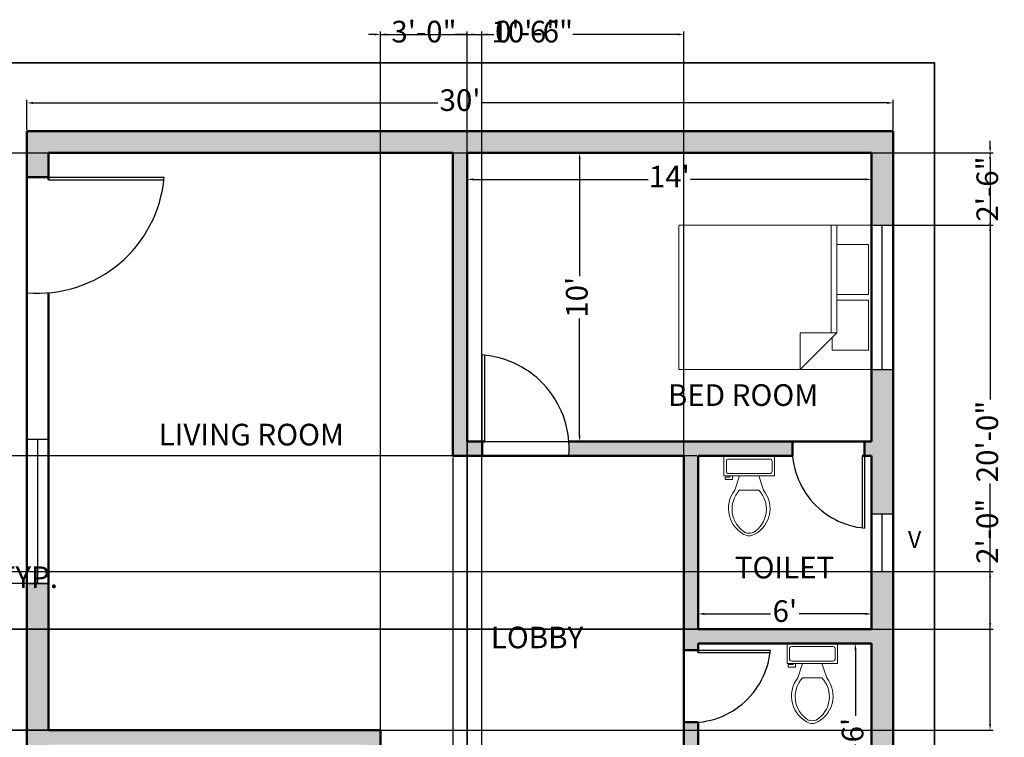
# Model space of a CAD drawing. Units: inches. Extents: x 2463 to 3327, y 6994 to 7582.
# Tile 5 of 5: x 2917 to 3327, y 7269 to 7567. Entities that reach past the tile are written whole.
import ezdxf

# ---------------------------------------------------------------- set-up
doc = ezdxf.new("R2010")
doc.units = ezdxf.units.IN
for name, color, linetype, lineweight in [('A-ANNO-DIMS', 2, 'Continuous', 18), ('A-ANNO-TEXT', 7, 'Continuous', 18), ('A-ANNO-TTLB', 7, 'Continuous', 35), ('A-AREA-IDEN', 3, 'Continuous', 25), ('A-DOOR', 4, 'Continuous', 25), ('A-FLOR-FIXT', 8, 'Continuous', 18), ('A-FURN', 8, 'Continuous', 18), ('A-GLAZ', 4, 'Continuous', 25), ('A-WALL', 7, 'Continuous', 50), ('A-WALL-PATT', 252, 'Continuous', 13)]:
    doc.layers.add(name, color=color, linetype=linetype, lineweight=lineweight)
doc.styles.get("Standard").update_dxf_attribs({"font": 'times.ttf'})
doc.dimstyles.new('ISO-25', dxfattribs={"dimtxt": 9, "dimasz": 2.5, "dimexe": 1.25, "dimexo": 0.625, "dimgap": 2, "dimtad": 0, "dimdec": 1, "dimlunit": 4, "dimtxsty": 'Standard', "dimcen": 2.5, "dimadec": 0, "dimazin": 0, "dimtfac": 1, "dimtdec": 1, "dimtmove": 0, "dimatfit": 3, "dimfxl": 1, "dimarcsym": 0})

# ---------------------------------------------------------------- blocks, each defined once
blk = doc.blocks.new('*D15')
at = {"layer": 'A-ANNO-DIMS', "color": 0, "lineweight": -2, "transparency": 16777216}
for p, q in [((3103.42, 7511.2), (3103.42, 7499.6)), ((3271.42, 7511.2), (3271.42, 7499.6)), ((3105.92, 7500.85), (3178.64, 7500.85)), ((3268.92, 7500.85), (3196.2, 7500.85))]:
    blk.add_line(p, q, dxfattribs=at)
at = {"layer": 'A-ANNO-DIMS', "color": 0, "transparency": 16777216}
for points in [[(3105.92, 7501.27), (3105.92, 7500.43), (3103.42, 7500.85)], [(3268.92, 7501.27), (3268.92, 7500.43), (3271.42, 7500.85)]]:
    blk.add_solid(points, dxfattribs=at)
at = {"layer": 'Defpoints', "color": 0, "transparency": 16777216}
for p in [(3103.42, 7511.83), (3271.42, 7511.83), (3271.42, 7500.85)]:
    blk.add_point(p, dxfattribs=at)
at = {"layer": 'A-ANNO-DIMS', "color": 0, "transparency": 16777216, "insert": (3187.42, 7500.85), "char_height": 9, "attachment_point": 5}
blk.add_mtext("14'", dxfattribs=at)
blk = doc.blocks.new('*D16')
at = {"layer": 'A-ANNO-DIMS', "color": 0, "lineweight": -2, "transparency": 16777216}
for p, q in [((3104.05, 7511.83), (3151.36, 7511.83)), ((3150.11, 7509.33), (3150.11, 7460.61)), ((3150.11, 7394.33), (3150.11, 7443.04)), ((3104.05, 7391.83), (3151.36, 7391.83))]:
    blk.add_line(p, q, dxfattribs=at)
at = {"layer": 'A-ANNO-DIMS', "color": 0, "transparency": 16777216}
for points in [[(3149.69, 7509.33), (3150.53, 7509.33), (3150.11, 7511.83)], [(3149.69, 7394.33), (3150.53, 7394.33), (3150.11, 7391.83)]]:
    blk.add_solid(points, dxfattribs=at)
at = {"layer": 'Defpoints', "color": 0, "transparency": 16777216}
for p in [(3103.42, 7511.83), (3103.42, 7391.83), (3150.11, 7391.83)]:
    blk.add_point(p, dxfattribs=at)
at = {"layer": 'A-ANNO-DIMS', "color": 0, "transparency": 16777216, "insert": (3150.11, 7451.83), "char_height": 9, "attachment_point": 5, "rotation": 90}
blk.add_mtext("10'", dxfattribs=at)
blk = doc.blocks.new('*D17')
at = {"layer": 'A-ANNO-DIMS', "color": 0, "lineweight": -2, "transparency": 16777216}
for p, q in [((3270.8, 7307.83), (3263.49, 7307.83)), ((3264.74, 7305.33), (3264.74, 7277.78)), ((3264.74, 7238.33), (3264.74, 7265.87)), ((3270.8, 7235.83), (3263.49, 7235.83))]:
    blk.add_line(p, q, dxfattribs=at)
at = {"layer": 'A-ANNO-DIMS', "color": 0, "transparency": 16777216}
for points in [[(3264.33, 7305.33), (3265.16, 7305.33), (3264.74, 7307.83)], [(3264.33, 7238.33), (3265.16, 7238.33), (3264.74, 7235.83)]]:
    blk.add_solid(points, dxfattribs=at)
at = {"layer": 'Defpoints', "color": 0, "transparency": 16777216}
for p in [(3264.74, 7307.83), (3271.42, 7307.83), (3271.42, 7235.83)]:
    blk.add_point(p, dxfattribs=at)
at = {"layer": 'A-ANNO-DIMS', "color": 0, "transparency": 16777216, "insert": (3264.74, 7271.83), "char_height": 9, "attachment_point": 5, "rotation": 90}
blk.add_mtext("6'", dxfattribs=at)
blk = doc.blocks.new('Bed - Queen')
for p, q in [((0, -80.00003), (0, 0)), ((0, 0), (59.99999, 0)), ((59.99999, 0), (59.99999, -80.00003)), ((7.99999, -1.2), (28.79998, -1.2)), ((7.99999, -14.4), (7.99999, -1.2)), ((28.79998, -1.2), (28.79998, -14.4)), ((31.19999, -1.2), (51.99999, -1.2)), ((31.19999, -14.4), (31.19999, -1.2)), ((51.99999, -1.2), (51.99999, -16.4)), ((0, -14.4), (44.8, -14.4)), ((59.99999, -29.6), (44.8, -14.4)), ((44.8, -14.4), (44.8, -29.6)), ((44.8, -16.8), (0, -16.8)), ((51.99999, -16.4), (46.79936, -16.4)), ((44.8, -29.6), (59.99999, -29.6)), ((59.99999, -80.00003), (0, -80.00003))]:
    blk.add_line(p, q)
blk = doc.blocks.new('*D18')
at = {"layer": 'A-ANNO-DIMS', "color": 0, "lineweight": -2, "transparency": 16777216}
for p, q in [((3199.42, 7314.45), (3199.42, 7321.4)), ((3271.42, 7314.45), (3271.42, 7321.4)), ((3201.92, 7320.15), (3229.47, 7320.15)), ((3268.92, 7320.15), (3241.37, 7320.15))]:
    blk.add_line(p, q, dxfattribs=at)
at = {"layer": 'A-ANNO-DIMS', "color": 0, "transparency": 16777216}
for points in [[(3201.92, 7320.57), (3201.92, 7319.73), (3199.42, 7320.15)], [(3268.92, 7320.57), (3268.92, 7319.73), (3271.42, 7320.15)]]:
    blk.add_solid(points, dxfattribs=at)
at = {"layer": 'Defpoints', "color": 0, "transparency": 16777216}
for p in [(3271.42, 7320.15), (3199.42, 7313.83), (3271.42, 7313.83)]:
    blk.add_point(p, dxfattribs=at)
at = {"layer": 'A-ANNO-DIMS', "color": 0, "transparency": 16777216, "insert": (3235.42, 7320.15), "char_height": 9, "attachment_point": 5}
blk.add_mtext("6'", dxfattribs=at)
blk = doc.blocks.new('*U11')
for p, q in [((9.5, -6), (9.5, -2)), ((-8, -8.5), (-8, -8)), ((-7, -8), (-7, -9.5)), ((-4, -8), (-6, -14)), ((4, -8), (6, -14)), ((-10, -8.5), (-8, -8.5)), ((-10, -9.5), (-10, -8.5)), ((-7, -9.5), (-10, -9.5)), ((4, -14), (-4, -14))]:
    blk.add_line(p, q)
blk.add_lwpolyline([(10.5, -8), (10.5, 0), (-10.5, 0), (-10.5, -8)], close=True)
for points in [[(-9.5, -2), (-9.5, -6)], [(8.5, -1), (-8.5, -1)], [(-8.5, -7), (8.5, -7)]]:
    blk.add_lwpolyline(points)
for centre, radius, start, end in [((-8.62, -1.88), 0.884, 81.8699, 188.1301), ((8.62, -1.88), 0.884, 351.8699, 98.1301), ((-8.62, -6.12), 0.884, 171.8699, 278.1301), ((8.62, -6.12), 0.884, 261.8699, 8.1301), ((3.52, -21.58), 12.17, 141.4691, 247.9714), ((4.2, -21.82), 11.33, 136.3677, 238.9468), ((-3.52, -21.58), 12.17, 292.0284, 38.5307), ((-4.2, -21.82), 11.33, 301.053, 43.6321), ((0, -27.88), 4, 245.7318, 294.2682), ((0, -29), 4, 254.8605, 285.1395)]:
    blk.add_arc(centre, radius, start, end)
blk = doc.blocks.new('*D25')
at = {"layer": 'A-ANNO-DIMS', "color": 0, "lineweight": -2, "transparency": 16777216}
for p, q in [((2920.42, 7521.45), (2920.42, 7533.89)), ((2922.92, 7532.64), (3091.13, 7532.64)), ((3277.92, 7532.64), (3109.71, 7532.64)), ((3280.42, 7521.45), (3280.42, 7533.89))]:
    blk.add_line(p, q, dxfattribs=at)
at = {"layer": 'A-ANNO-DIMS', "color": 0, "transparency": 16777216}
for points in [[(2922.92, 7533.06), (2922.92, 7532.22), (2920.42, 7532.64)], [(3277.92, 7533.06), (3277.92, 7532.22), (3280.42, 7532.64)]]:
    blk.add_solid(points, dxfattribs=at)
at = {"layer": 'Defpoints', "color": 0, "transparency": 16777216}
for p in [(3280.42, 7532.64), (2920.42, 7520.83), (3280.42, 7520.83)]:
    blk.add_point(p, dxfattribs=at)
at = {"layer": 'A-ANNO-DIMS', "color": 0, "transparency": 16777216, "insert": (3100.42, 7532.64), "char_height": 9, "attachment_point": 5}
blk.add_mtext("30'", dxfattribs=at)
blk = doc.blocks.new('DOOR-36')
for p, q in [((0, 6), (0, 42)), ((1, 6), (1, 41.91))]:
    blk.add_line(p, q)
blk.add_arc((-3, 3), 39.12, 355.6013, 85.6013)
blk = doc.blocks.new('DOOR-30')
for p, q in [((29.14, 30), (29.14, 0)), ((30.14, 30), (30.14, 0))]:
    blk.add_line(p, q)
blk.add_arc((33.14, 33), 33.14, 174.8056, 264.8056)
blk = doc.blocks.new('DOOR-48')
for p, q in [((9, 48.19), (57, 48.19)), ((9, 47.19), (56.91, 47.19))]:
    blk.add_line(p, q)
blk.add_arc((4.5, 52.69), 52.69, 265.1009, 355.1009)
blk = doc.blocks.new('WIN-60')
for p, q in [((9, 60), (0, 60)), ((4.5, 60), (4.5, 0)), ((9, 0), (0, 0))]:
    blk.add_line(p, q)
blk = doc.blocks.new('WIN-24')
for p, q in [((9, 24), (0, 24)), ((4.5, 24), (4.5, 0)), ((9, 0), (0, 0))]:
    blk.add_line(p, q)
blk = doc.blocks.new('*D40')
at = {"layer": 'A-ANNO-DIMS', "color": 0, "lineweight": -2, "transparency": 16777216}
for p, q in [((2864.43, 7337.2), (2864.43, 7332.98)), ((2866.93, 7334.23), (2870.93, 7334.23)), ((2873.43, 7337.2), (2873.43, 7332.98)), ((2873.43, 7334.23), (2875.93, 7334.23))]:
    blk.add_line(p, q, dxfattribs=at)
at = {"layer": 'A-ANNO-DIMS', "color": 0, "transparency": 16777216}
for points in [[(2866.93, 7334.64), (2866.93, 7333.81), (2864.43, 7334.23)], [(2870.93, 7334.64), (2870.93, 7333.81), (2873.43, 7334.23)]]:
    blk.add_solid(points, dxfattribs=at)
at = {"layer": 'Defpoints', "color": 0, "transparency": 16777216}
for p in [(2864.43, 7337.83), (2873.43, 7337.83), (2873.43, 7334.23)]:
    blk.add_point(p, dxfattribs=at)
at = {"layer": 'A-ANNO-DIMS', "color": 0, "transparency": 16777216, "insert": (2905.86, 7334.23), "char_height": 9, "attachment_point": 5}
blk.add_mtext('0\'-9" TYP.', dxfattribs=at)
blk = doc.blocks.new('*D51')
at = {"layer": 'A-ANNO-DIMS', "color": 0, "lineweight": -2, "transparency": 16777216}
for p, q in [((2523.06, 7511.83), (3321.97, 7511.83)), ((3320.72, 7509.33), (3320.72, 7409.33)), ((3320.72, 7274.33), (3320.72, 7374.32)), ((2523.06, 7271.83), (3321.97, 7271.83))]:
    blk.add_line(p, q, dxfattribs=at)
at = {"layer": 'A-ANNO-DIMS', "color": 0, "transparency": 16777216}
for points in [[(3320.31, 7509.33), (3321.14, 7509.33), (3320.72, 7511.83)], [(3320.31, 7274.33), (3321.14, 7274.33), (3320.72, 7271.83)]]:
    blk.add_solid(points, dxfattribs=at)
at = {"layer": 'Defpoints', "color": 0, "transparency": 16777216}
for p in [(2522.43, 7511.83), (2522.43, 7271.83), (3320.72, 7271.83)]:
    blk.add_point(p, dxfattribs=at)
at = {"layer": 'A-ANNO-DIMS', "color": 0, "transparency": 16777216, "insert": (3320.72, 7391.83), "char_height": 9, "attachment_point": 5, "rotation": 90}
blk.add_mtext('20\'-0"', dxfattribs=at)
blk = doc.blocks.new('*D65')
at = {"layer": 'A-ANNO-DIMS', "color": 0, "lineweight": -2, "transparency": 16777216}
for p, q in [((2865.06, 7337.83), (3321.97, 7337.83)), ((3320.72, 7337.83), (3320.72, 7340.33)), ((3320.72, 7316.33), (3320.72, 7335.33)), ((2865.06, 7313.83), (3321.97, 7313.83))]:
    blk.add_line(p, q, dxfattribs=at)
at = {"layer": 'A-ANNO-DIMS', "color": 0, "transparency": 16777216}
for points in [[(3320.31, 7335.33), (3321.14, 7335.33), (3320.72, 7337.83)], [(3320.31, 7316.33), (3321.14, 7316.33), (3320.72, 7313.83)]]:
    blk.add_solid(points, dxfattribs=at)
at = {"layer": 'Defpoints', "color": 0, "transparency": 16777216}
for p in [(2864.43, 7337.83), (3320.72, 7337.83), (2864.43, 7313.83)]:
    blk.add_point(p, dxfattribs=at)
at = {"layer": 'A-ANNO-DIMS', "color": 0, "transparency": 16777216, "insert": (3320.72, 7354.51), "char_height": 9, "attachment_point": 5, "rotation": 90}
blk.add_mtext('2\'-0"', dxfattribs=at)
blk = doc.blocks.new('*D68')
at = {"layer": 'A-ANNO-DIMS', "color": 0, "lineweight": -2, "transparency": 16777216}
for p, q in [((3103.42, 7391.2), (3103.42, 6999.28)), ((3097.42, 7385.2), (3097.42, 6999.28)), ((3094.92, 7000.53), (3092.42, 7000.53)), ((3097.42, 7000.53), (3103.42, 7000.53)), ((3105.92, 7000.53), (3108.42, 7000.53))]:
    blk.add_line(p, q, dxfattribs=at)
at = {"layer": 'A-ANNO-DIMS', "color": 0, "transparency": 16777216}
for points in [[(3094.92, 7000.94), (3094.92, 7000.11), (3097.42, 7000.53)], [(3105.92, 7000.94), (3105.92, 7000.11), (3103.42, 7000.53)]]:
    blk.add_solid(points, dxfattribs=at)
at = {"layer": 'Defpoints', "color": 0, "transparency": 16777216}
for p in [(3103.42, 7391.83), (3097.42, 7385.83), (3103.42, 7000.53)]:
    blk.add_point(p, dxfattribs=at)
at = {"layer": 'A-ANNO-DIMS', "color": 0, "transparency": 16777216, "insert": (3122.51, 7000.53), "char_height": 9, "attachment_point": 5}
blk.add_mtext('0\'-6"', dxfattribs=at)
blk = doc.blocks.new('*D69')
at = {"layer": 'A-ANNO-DIMS', "color": 0, "lineweight": -2, "transparency": 16777216}
for p, q in [((3198.8, 7385.83), (2471.88, 7385.83)), ((2473.13, 7383.33), (2473.13, 7363.87)), ((2473.13, 7316.33), (2473.13, 7335.79)), ((3198.8, 7313.83), (2471.88, 7313.83))]:
    blk.add_line(p, q, dxfattribs=at)
at = {"layer": 'A-ANNO-DIMS', "color": 0, "transparency": 16777216}
for points in [[(2472.71, 7383.33), (2473.55, 7383.33), (2473.13, 7385.83)], [(2472.71, 7316.33), (2473.55, 7316.33), (2473.13, 7313.83)]]:
    blk.add_solid(points, dxfattribs=at)
at = {"layer": 'Defpoints', "color": 0, "transparency": 16777216}
for p in [(3199.42, 7385.83), (2473.13, 7313.83), (3199.42, 7313.83)]:
    blk.add_point(p, dxfattribs=at)
at = {"layer": 'A-ANNO-DIMS', "color": 0, "transparency": 16777216, "insert": (2473.13, 7349.83), "char_height": 9, "attachment_point": 5, "rotation": 90}
blk.add_mtext('6\'-0"', dxfattribs=at)
blk = doc.blocks.new('*D70')
at = {"layer": 'A-ANNO-DIMS', "color": 0, "lineweight": -2, "transparency": 16777216}
for p, q in [((2930.05, 7511.83), (3321.97, 7511.83)), ((3320.72, 7509.33), (3320.72, 7409.33)), ((3320.72, 7274.33), (3320.72, 7374.32)), ((2930.05, 7271.83), (3321.97, 7271.83))]:
    blk.add_line(p, q, dxfattribs=at)
at = {"layer": 'A-ANNO-DIMS', "color": 0, "transparency": 16777216}
for points in [[(3320.31, 7509.33), (3321.14, 7509.33), (3320.72, 7511.83)], [(3320.31, 7274.33), (3321.14, 7274.33), (3320.72, 7271.83)]]:
    blk.add_solid(points, dxfattribs=at)
at = {"layer": 'Defpoints', "color": 0, "transparency": 16777216}
for p in [(2929.42, 7511.83), (2929.42, 7271.83), (3320.72, 7271.83)]:
    blk.add_point(p, dxfattribs=at)
at = {"layer": 'A-ANNO-DIMS', "color": 0, "transparency": 16777216, "insert": (3320.72, 7391.83), "char_height": 9, "attachment_point": 5, "rotation": 90}
blk.add_mtext('20\'-0"', dxfattribs=at)
blk = doc.blocks.new('*D71')
at = {"layer": 'A-ANNO-DIMS', "color": 0, "lineweight": -2, "transparency": 16777216}
for p, q in [((3067.42, 7272.45), (3067.42, 7562.38)), ((3069.92, 7561.13), (3113.55, 7561.13)), ((3190.92, 7561.13), (3147.29, 7561.13)), ((3193.42, 7230.45), (3193.42, 7562.38))]:
    blk.add_line(p, q, dxfattribs=at)
at = {"layer": 'A-ANNO-DIMS', "color": 0, "transparency": 16777216}
for points in [[(3069.92, 7561.54), (3069.92, 7560.71), (3067.42, 7561.13)], [(3190.92, 7561.54), (3190.92, 7560.71), (3193.42, 7561.13)]]:
    blk.add_solid(points, dxfattribs=at)
at = {"layer": 'Defpoints', "color": 0, "transparency": 16777216}
for p in [(3193.42, 7561.13), (3067.42, 7271.83), (3193.42, 7229.83)]:
    blk.add_point(p, dxfattribs=at)
at = {"layer": 'A-ANNO-DIMS', "color": 0, "transparency": 16777216, "insert": (3130.42, 7561.13), "char_height": 9, "attachment_point": 5}
blk.add_mtext('10\'-6"', dxfattribs=at)
blk = doc.blocks.new('*D73')
at = {"layer": 'A-ANNO-DIMS', "color": 0, "lineweight": -2, "transparency": 16777216}
for p, q in [((3064.92, 7561.13), (3062.42, 7561.13)), ((3067.42, 7180.45), (3067.42, 7562.38)), ((3067.42, 7561.13), (3071.37, 7561.13)), ((3103.42, 7561.13), (3099.48, 7561.13)), ((3103.42, 7190.45), (3103.42, 7562.38)), ((3105.92, 7561.13), (3108.42, 7561.13))]:
    blk.add_line(p, q, dxfattribs=at)
at = {"layer": 'A-ANNO-DIMS', "color": 0, "transparency": 16777216}
for points in [[(3064.92, 7561.54), (3064.92, 7560.71), (3067.42, 7561.13)], [(3105.92, 7561.54), (3105.92, 7560.71), (3103.42, 7561.13)]]:
    blk.add_solid(points, dxfattribs=at)
at = {"layer": 'Defpoints', "color": 0, "transparency": 16777216}
for p in [(3103.42, 7561.13), (3103.42, 7189.83), (3067.42, 7179.83)]:
    blk.add_point(p, dxfattribs=at)
at = {"layer": 'A-ANNO-DIMS', "color": 0, "transparency": 16777216, "insert": (3085.42, 7561.13), "char_height": 9, "attachment_point": 5}
blk.add_mtext('3\'-0"', dxfattribs=at)
blk = doc.blocks.new('*D74')
at = {"layer": 'A-ANNO-DIMS', "color": 0, "lineweight": -2, "transparency": 16777216}
for p, q in [((3100.92, 7561.13), (3098.42, 7561.13)), ((3103.42, 7190.45), (3103.42, 7562.38)), ((3103.42, 7561.13), (3109.42, 7561.13)), ((3109.42, 7190.45), (3109.42, 7562.38)), ((3111.92, 7561.13), (3114.42, 7561.13))]:
    blk.add_line(p, q, dxfattribs=at)
at = {"layer": 'A-ANNO-DIMS', "color": 0, "transparency": 16777216}
for points in [[(3100.92, 7561.54), (3100.92, 7560.71), (3103.42, 7561.13)], [(3111.92, 7561.54), (3111.92, 7560.71), (3109.42, 7561.13)]]:
    blk.add_solid(points, dxfattribs=at)
at = {"layer": 'Defpoints', "color": 0, "transparency": 16777216}
for p in [(3109.42, 7561.13), (3103.42, 7189.83), (3109.42, 7189.83)]:
    blk.add_point(p, dxfattribs=at)
at = {"layer": 'A-ANNO-DIMS', "color": 0, "transparency": 16777216, "insert": (3128.51, 7561.13), "char_height": 9, "attachment_point": 5}
blk.add_mtext('0\'-6"', dxfattribs=at)
blk = doc.blocks.new('*D78')
at = {"layer": 'A-ANNO-DIMS', "color": 0, "lineweight": -2, "transparency": 16777216}
for p, q in [((2928.8, 7332.77), (2471.88, 7332.77)), ((2473.13, 7330.27), (2473.13, 7316.3)), ((2473.13, 7274.33), (2473.13, 7288.29)), ((2928.8, 7271.83), (2471.88, 7271.83))]:
    blk.add_line(p, q, dxfattribs=at)
at = {"layer": 'A-ANNO-DIMS', "color": 0, "transparency": 16777216}
for points in [[(2472.71, 7330.27), (2473.55, 7330.27), (2473.13, 7332.77)], [(2472.71, 7274.33), (2473.55, 7274.33), (2473.13, 7271.83)]]:
    blk.add_solid(points, dxfattribs=at)
at = {"layer": 'Defpoints', "color": 0, "transparency": 16777216}
for p in [(2473.13, 7332.77), (2929.42, 7332.77), (2929.42, 7271.83)]:
    blk.add_point(p, dxfattribs=at)
at = {"layer": 'A-ANNO-DIMS', "color": 0, "transparency": 16777216, "insert": (2473.13, 7302.3), "char_height": 9, "attachment_point": 5, "rotation": 90}
blk.add_mtext('5\'-1"', dxfattribs=at)
blk = doc.blocks.new('*D79')
at = {"layer": 'A-ANNO-DIMS', "color": 0, "lineweight": -2, "transparency": 16777216}
for p, q in [((3320.72, 7514.33), (3320.72, 7516.83)), ((3272.05, 7511.83), (3321.97, 7511.83)), ((3320.72, 7511.83), (3320.72, 7511.01)), ((3272.05, 7481.83), (3321.97, 7481.83)), ((3320.72, 7481.83), (3320.72, 7482.64)), ((3320.72, 7479.33), (3320.72, 7476.83))]:
    blk.add_line(p, q, dxfattribs=at)
at = {"layer": 'A-ANNO-DIMS', "color": 0, "transparency": 16777216}
for points in [[(3320.31, 7514.33), (3321.14, 7514.33), (3320.72, 7511.83)], [(3320.31, 7479.33), (3321.14, 7479.33), (3320.72, 7481.83)]]:
    blk.add_solid(points, dxfattribs=at)
at = {"layer": 'Defpoints', "color": 0, "transparency": 16777216}
for p in [(3271.42, 7511.83), (3271.42, 7481.83), (3320.72, 7481.83)]:
    blk.add_point(p, dxfattribs=at)
at = {"layer": 'A-ANNO-DIMS', "color": 0, "transparency": 16777216, "insert": (3320.72, 7496.83), "char_height": 9, "attachment_point": 5, "rotation": 90}
blk.add_mtext('2\'-6"', dxfattribs=at)
blk = doc.blocks.new('*D80')
at = {"layer": 'A-ANNO-DIMS', "color": 0, "lineweight": -2, "transparency": 16777216}
for p, q in [((3272.05, 7337.83), (3321.97, 7337.83)), ((3320.72, 7337.83), (3320.72, 7340.33)), ((3320.72, 7316.33), (3320.72, 7335.33)), ((3272.05, 7313.83), (3321.97, 7313.83))]:
    blk.add_line(p, q, dxfattribs=at)
at = {"layer": 'A-ANNO-DIMS', "color": 0, "transparency": 16777216}
for points in [[(3320.31, 7335.33), (3321.14, 7335.33), (3320.72, 7337.83)], [(3320.31, 7316.33), (3321.14, 7316.33), (3320.72, 7313.83)]]:
    blk.add_solid(points, dxfattribs=at)
at = {"layer": 'Defpoints', "color": 0, "transparency": 16777216}
for p in [(3271.42, 7337.83), (3320.72, 7337.83), (3271.42, 7313.83)]:
    blk.add_point(p, dxfattribs=at)
at = {"layer": 'A-ANNO-DIMS', "color": 0, "transparency": 16777216, "insert": (3320.72, 7354.51), "char_height": 9, "attachment_point": 5, "rotation": 90}
blk.add_mtext('2\'-0"', dxfattribs=at)

msp = doc.modelspace()

# ---------------------------------------------------------------- hatches: boundary and pattern name
at = {"layer": 'A-WALL-PATT'}
h = msp.add_hatch(color=256, dxfattribs=at)
h.dxf.hatch_style = 1
h.paths.add_polyline_path([(2522.43, 7511.83), (2690.43, 7511.83), (2690.43, 7385.83), (2696.43, 7385.83), (2702.68, 7385.83), (2702.68, 7391.83), (2696.43, 7391.83), (2696.43, 7511.83), (2864.43, 7511.83), (2864.43, 7481.83), (2873.43, 7481.83), (2873.43, 7520.83), (2513.43, 7520.83), (2513.43, 7501.71), (2522.43, 7501.71)])
h.paths.add_polyline_path([(2522.43, 7453.71, -0.042779), (2513.43, 7453.71), (2513.43, 7392.77), (2522.43, 7392.77)], flags=0)
h.paths.add_polyline_path([(2522.43, 7332.77), (2513.43, 7332.77), (2513.43, 7226.83), (2522.43, 7226.83), (2522.43, 7265.83), (2654.43, 7265.83), (2654.43, 7263.42), (2660.43, 7263.42), (2660.43, 7271.83), (2522.43, 7271.83)])
h.paths.add_polyline_path([(2873.43, 7421.83), (2864.43, 7421.83), (2864.43, 7391.83), (2861.59, 7391.83), (2861.59, 7385.83), (2864.43, 7385.83), (2864.43, 7361.83), (2873.43, 7361.83)])
h.paths.add_polyline_path([(2792.43, 7385.83), (2831.59, 7385.83, -0.045361), (2831.59, 7391.83), (2738.68, 7391.83, -0.038405), (2738.68, 7385.83), (2786.43, 7385.83), (2786.43, 7313.83), (2786.43, 7307.83), (2786.43, 7305.07), (2792.43, 7305.07), (2792.43, 7307.83), (2864.43, 7307.83), (2864.43, 7235.83), (2792.43, 7235.83), (2792.43, 7275.07, -0.045361), (2786.43, 7275.07), (2786.43, 7235.83), (2786.43, 7229.83), (2864.43, 7229.83), (2864.43, 7169.83), (2873.43, 7169.83), (2873.43, 7337.83), (2864.43, 7337.83), (2864.43, 7313.83), (2792.43, 7313.83)])
h.paths.add_polyline_path([(2873.43, 7109.83), (2864.43, 7109.83), (2864.43, 7049.83), (2834.43, 7049.83), (2834.43, 7040.83), (2873.43, 7040.83)])
h.paths.add_polyline_path([(2774.43, 7049.83), (2744.43, 7049.83), (2744.43, 7199.83), (2738.43, 7199.83), (2738.43, 7049.83), (2723.43, 7049.83), (2723.43, 7040.83), (2774.43, 7040.83)])
h.paths.add_polyline_path([(2675.43, 7049.83), (2660.43, 7049.83), (2660.43, 7121.83), (2660.43, 7127.83), (2660.43, 7227.42, -0.038405), (2654.43, 7227.42), (2654.43, 7127.83), (2651.08, 7127.83), (2651.08, 7121.83), (2654.43, 7121.83), (2654.43, 7049.83), (2522.43, 7049.83), (2522.43, 7073.83), (2513.43, 7073.83), (2513.43, 7040.83), (2675.43, 7040.83)])
h.paths.add_polyline_path([(2621.08, 7127.83), (2522.43, 7127.83), (2522.43, 7166.83), (2513.43, 7166.83), (2513.43, 7097.83), (2522.43, 7097.83), (2522.43, 7121.83), (2621.08, 7121.83, -0.045361)], flags=17)
h.paths.add_polyline_path([(3280.42, 7520.83), (2920.42, 7520.83), (2920.42, 7501.71), (2929.42, 7501.71), (2929.42, 7511.83), (3097.42, 7511.83), (3097.42, 7385.83), (3103.42, 7385.83), (3109.67, 7385.83), (3109.67, 7391.83), (3103.42, 7391.83), (3103.42, 7511.83), (3271.42, 7511.83), (3271.42, 7481.83), (3280.42, 7481.83)])
h.paths.add_polyline_path([(3280.42, 7421.83), (3271.42, 7421.83), (3271.42, 7391.83), (3268.58, 7391.83), (3268.58, 7385.83), (3271.42, 7385.83), (3271.42, 7361.83), (3280.42, 7361.83)])
h.paths.add_polyline_path([(3238.58, 7391.83), (3145.67, 7391.83, -0.038405), (3145.67, 7385.83), (3193.42, 7385.83), (3193.42, 7313.83), (3193.42, 7307.83), (3193.42, 7305.07), (3199.42, 7305.07), (3199.42, 7307.83), (3271.42, 7307.83), (3271.42, 7235.83), (3199.42, 7235.83), (3193.42, 7235.83), (3193.42, 7229.83), (3271.42, 7229.83), (3280.42, 7229.83), (3280.42, 7337.83), (3271.42, 7337.83), (3271.42, 7313.83), (3199.42, 7313.83), (3199.42, 7385.83), (3238.58, 7385.83, -0.045361)])
h.paths.add_polyline_path([(3199.42, 7275.07, -0.045361), (3193.42, 7275.07), (3193.42, 7235.83), (3199.42, 7235.83)], flags=17)
h.paths.add_polyline_path([(3193.42, 7235.83), (3145.42, 7235.83), (3145.42, 7227.44), (3151.42, 7227.44), (3151.42, 7229.83), (3193.42, 7229.83)])
h.paths.add_polyline_path([(3151.42, 7199.83, -0.044871), (3145.42, 7199.83), (3145.42, 7049.83), (3130.42, 7049.83), (3130.42, 7040.83), (3151.42, 7040.83), (3151.42, 7049.83)])
h.paths.add_polyline_path([(3082.42, 7049.83), (3067.42, 7049.83), (3067.42, 7121.83), (3067.42, 7127.83), (3067.42, 7227.42, -0.038405), (3061.42, 7227.42), (3061.42, 7127.83), (3058.07, 7127.83), (3058.07, 7121.83), (3061.42, 7121.83), (3061.42, 7049.83), (2929.42, 7049.83), (2929.42, 7073.83), (2920.42, 7073.83), (2920.42, 7040.83), (3082.42, 7040.83)])
h.paths.add_polyline_path([(3028.07, 7121.83), (2997.56, 7121.83), (2997.56, 7113.83), (2991.06, 7113.83), (2993.06, 7107.83, -0.501323), (2988.1, 7088.96, -0.132891), (2986.01, 7088.96, -0.501317), (2981.06, 7107.83), (2983.06, 7113.83), (2980.06, 7113.83), (2980.06, 7112.33), (2977.06, 7112.33), (2977.06, 7113.83), (2976.56, 7113.83), (2976.56, 7121.83), (2929.42, 7121.83), (2929.42, 7097.83), (2920.42, 7097.83), (2920.42, 7166.83), (2929.42, 7166.83), (2929.42, 7127.83), (3028.07, 7127.83, 0.045361)], flags=17)
h.paths.add_polyline_path([(2995.56, 7120.83, -0.414214), (2996.56, 7120.08), (2996.56, 7115.83, -0.414214), (2995.81, 7114.83), (2978.56, 7114.83, -0.414214), (2977.56, 7115.58), (2977.56, 7119.83, -0.414214), (2978.31, 7120.83)], flags=16)
h.paths.add_polyline_path([(2988.7, 7090.3, -0.215004), (2985.41, 7090.3, -0.48008), (2983.06, 7107.83), (2991.06, 7107.83, -0.48008)], flags=16)
h.paths.add_polyline_path([(2929.42, 7265.83), (3061.42, 7265.83), (3061.42, 7263.42), (3067.42, 7263.42), (3067.42, 7271.83), (2929.42, 7271.83), (2929.42, 7332.77), (2920.42, 7332.77), (2920.42, 7226.83), (2929.42, 7226.83)])
h.paths.add_polyline_path([(2929.42, 7453.71, -0.042779), (2920.42, 7453.71), (2920.42, 7392.77), (2929.42, 7392.77)], flags=0)

# ---------------------------------------------------------------- linework, layer by layer
at = {"layer": 'A-ANNO-TTLB'}
msp.add_lwpolyline([(2463.47, 7549.29), (3297.67, 7549.29), (3297.67, 7021.48), (2463.47, 7021.48)], close=True, dxfattribs=at)
at = {"layer": 'A-WALL'}
for p, q in [((2920.42, 7520.83), (3280.42, 7520.83)), ((2920.42, 7040.83), (2920.42, 7520.83)), ((3280.42, 7520.83), (3280.42, 7040.83)), ((2929.42, 7511.83), (3097.42, 7511.83)), ((2929.42, 7501.71), (2929.42, 7511.83)), ((3097.42, 7511.83), (3097.42, 7385.83)), ((3103.42, 7511.83), (3271.42, 7511.83)), ((3103.42, 7511.83), (3103.42, 7391.83)), ((3271.42, 7511.83), (3271.42, 7391.83)), ((2929.42, 7501.71), (2920.42, 7501.71)), ((2929.42, 7500.71), (2929.42, 7501.71)), ((2929.42, 7271.83), (2929.42, 7453.71)), ((3103.42, 7391.83), (3110.67, 7391.83)), ((3109.67, 7391.83), (3109.67, 7385.83)), ((3145.67, 7391.83), (3271.42, 7391.83)), ((3238.58, 7385.83), (3238.58, 7391.83)), ((3268.58, 7385.83), (3268.58, 7391.83)), ((3103.42, 7385.83), (3097.42, 7385.83)), ((3103.42, 7385.83), (3193.42, 7385.83)), ((3193.42, 7385.83), (3193.42, 7313.83)), ((3199.42, 7385.83), (3238.58, 7385.83)), ((3199.42, 7385.83), (3199.42, 7313.83)), ((3267.58, 7385.83), (3271.42, 7385.83)), ((3271.42, 7385.83), (3271.42, 7313.83)), ((3193.42, 7313.83), (3193.42, 7307.83)), ((3199.42, 7313.83), (3271.42, 7313.83)), ((3193.42, 7307.83), (3193.42, 7235.83)), ((3199.42, 7305.07), (3193.42, 7305.07)), ((3199.42, 7307.83), (3271.42, 7307.83)), ((3199.42, 7307.83), (3199.42, 7304.07)), ((3271.42, 7307.83), (3271.42, 7235.83)), ((3199.42, 7275.07), (3193.42, 7275.07)), ((3199.42, 7275.07), (3199.42, 7235.83)), ((3067.42, 7271.83), (2929.42, 7271.83)), ((3067.42, 7127.83), (3067.42, 7271.83))]:
    msp.add_line(p, q, dxfattribs=at)

# ---------------------------------------------------------------- block references
at = {"layer": 'A-DOOR'}
for name, p in [('DOOR-48', (2920.42, 7453.52)), ('DOOR-36', (3109.67, 7385.83)), ('DOOR-30', (3238.45, 7355.83))]:
    msp.add_blockref(name, p, dxfattribs=at)
at = {"layer": 'A-DOOR', "rotation": 90.02301063229471}
msp.add_blockref('DOOR-30', (3229.42, 7274.94), dxfattribs=at)
at = {"layer": 'A-FLOR-FIXT'}
for p in [(3220.61, 7385.55), (3246.82, 7307.55)]:
    msp.add_blockref('*U11', p, dxfattribs=at)
at = {"layer": 'A-FURN', "rotation": 270}
msp.add_blockref('Bed - Queen', (3271.42, 7481.83), dxfattribs=at)
at = {"layer": 'A-GLAZ', "rotation": 180}
for name, p in [('WIN-60', (3280.42, 7481.83)), ('WIN-60', (2929.42, 7392.77)), ('WIN-24', (3280.42, 7361.83))]:
    msp.add_blockref(name, p, dxfattribs=at)

# ---------------------------------------------------------------- texts
at = {"layer": 'A-ANNO-TEXT', "insert": (3275.15, 7354.57), "char_height": 7, "attachment_point": 1}
msp.add_mtext_dynamic_manual_height_columns('\\pxqc;{\\fTimes New Roman|b1|i0|c0|p18;V}', width=28.3852, gutter_width=12.5, heights=[0], dxfattribs=at)
at = {"layer": 'A-AREA-IDEN', "char_height": 9, "attachment_point": 1}
for s, width, insert in [('\\pxqc;{\\fTimes New Roman|b1|i0|c0|p18;BED ROOM}', 86.127, (3175, 7415.64)), ('\\pxqc;{\\fTimes New Roman|b1|i0|c0|p18;LIVING ROOM}', 122.533, (2952.42, 7399.21)), ('\\pxqc;{\\fTimes New Roman|b1|i0|c0|p18;TOILET}', 62.7452, (3203.92, 7343.91)), ('\\pxqc;{\\fTimes New Roman|b1|i0|c0|p18;LOBBY}', 90.7623, (3087.04, 7314.86))]:
    msp.add_mtext_dynamic_manual_height_columns(s, width=width, gutter_width=12.5, heights=[0], dxfattribs=dict(at, insert=insert))

# ---------------------------------------------------------------- dimensions: what is measured, and where the dimension line sits
at = {"layer": 'A-ANNO-DIMS'}
for base, p1, p2, override, picture, middle in [((3103.42, 7561.13), (3067.42, 7179.83), (3103.42, 7189.83), {"dimdec": 1, "dimlfac": 1, "dimrnd": 0, "dimzin": 1, "dimdsep": 46, "dimlunit": 4, "dimfrac": 2}, '*D73', (3085.42, 7561.13)), ((3193.42, 7561.13), (3067.42, 7271.83), (3193.42, 7229.83), {"dimdec": 1, "dimlfac": 1, "dimrnd": 0, "dimzin": 1, "dimdsep": 46, "dimlunit": 4, "dimfrac": 2}, '*D71', (3130.42, 7561.13)), ((3109.42, 7561.13), (3103.42, 7189.83), (3109.42, 7189.83), {"dimdec": 1, "dimlfac": 1, "dimrnd": 0, "dimzin": 1, "dimdsep": 46, "dimlunit": 4, "dimfrac": 2}, '*D74', (3128.51, 7561.13)), ((3280.42, 7532.64), (2920.42, 7520.83), (3280.42, 7520.83), {"dimclrd": 0, "dimclre": 0, "dimclrt": 0}, '*D25', (3100.42, 7532.64)), ((3271.42, 7500.85), (3103.42, 7511.83), (3271.42, 7511.83), {"dimclrd": 0, "dimclre": 0, "dimclrt": 0}, '*D15', (3187.42, 7500.85)), ((3103.42, 7000.53), (3097.42, 7385.83), (3103.42, 7391.83), {"dimdec": 1, "dimlfac": 1, "dimrnd": 0, "dimzin": 1, "dimdsep": 46, "dimlunit": 4, "dimfrac": 2}, '*D68', (3122.51, 7000.53)), ((3271.42, 7320.15), (3199.42, 7313.83), (3271.42, 7313.83), {"dimclrd": 0, "dimclre": 0, "dimclrt": 0}, '*D18', (3235.42, 7320.15))]:
    dim = msp.add_linear_dim(base=base, p1=p1, p2=p2, dimstyle='ISO-25', override=override, dxfattribs=at)
    dim.commit()
    dim.dimension.update_dxf_attribs({"geometry": picture, "text_midpoint": middle})
for base, p1, p2, override, picture, middle in [((3320.72, 7481.83), (3271.42, 7511.83), (3271.42, 7481.83), {"dimdec": 1, "dimlfac": 1, "dimrnd": 0, "dimzin": 1, "dimdsep": 46, "dimlunit": 4, "dimfrac": 2}, '*D79', (3320.72, 7496.83)), ((3320.72, 7271.83), (2522.43, 7511.83), (2522.43, 7271.83), {"dimdec": 1, "dimlfac": 1, "dimrnd": 0, "dimzin": 1, "dimdsep": 46, "dimlunit": 4, "dimfrac": 2}, '*D51', (3320.72, 7391.83)), ((3320.72, 7271.83), (2929.42, 7511.83), (2929.42, 7271.83), {"dimdec": 1, "dimlfac": 1, "dimrnd": 0, "dimzin": 1, "dimdsep": 46, "dimlunit": 4, "dimfrac": 2}, '*D70', (3320.72, 7391.83)), ((3150.11, 7391.83), (3103.42, 7511.83), (3103.42, 7391.83), {"dimclrd": 0, "dimclre": 0, "dimclrt": 0}, '*D16', (3150.11, 7451.83)), ((2473.13, 7313.83), (3199.42, 7385.83), (3199.42, 7313.83), {"dimdec": 1, "dimlfac": 1, "dimrnd": 0, "dimzin": 1, "dimdsep": 46, "dimlunit": 4, "dimfrac": 2}, '*D69', (2473.13, 7349.83)), ((3320.72, 7337.83), (2864.43, 7313.83), (2864.43, 7337.83), {"dimdec": 1, "dimlfac": 1, "dimrnd": 0, "dimzin": 1, "dimdsep": 46, "dimlunit": 4, "dimfrac": 2}, '*D65', (3320.72, 7354.51)), ((3320.72, 7337.83), (3271.42, 7313.83), (3271.42, 7337.83), {"dimdec": 1, "dimlfac": 1, "dimrnd": 0, "dimzin": 1, "dimdsep": 46, "dimlunit": 4, "dimfrac": 2}, '*D80', (3320.72, 7354.51)), ((2473.13, 7332.77), (2929.42, 7271.83), (2929.42, 7332.77), {"dimdec": 1, "dimlfac": 1, "dimrnd": 0, "dimzin": 1, "dimdsep": 46, "dimlunit": 4, "dimfrac": 2}, '*D78', (2473.13, 7302.3)), ((3264.74, 7307.83), (3271.42, 7235.83), (3271.42, 7307.83), {"dimclrd": 0, "dimclre": 0, "dimclrt": 0}, '*D17', (3264.74, 7271.83))]:
    dim = msp.add_linear_dim(base=base, p1=p1, p2=p2, angle=90, dimstyle='ISO-25', override=override, dxfattribs=at)
    dim.commit()
    dim.dimension.update_dxf_attribs({"geometry": picture, "text_midpoint": middle})
dim = msp.add_linear_dim(base=(2873.43, 7334.23), p1=(2864.43, 7337.83), p2=(2873.43, 7337.83), text='<> TYP.', dimstyle='ISO-25', override={"dimdec": 1, "dimrnd": 0, "dimzin": 1, "dimlunit": 4, "dimfrac": 2}, dxfattribs=at)
dim.commit()
dim.dimension.update_dxf_attribs({"geometry": '*D40', "text_midpoint": (2905.86, 7334.23)})

doc.saveas('drawing.dxf')
